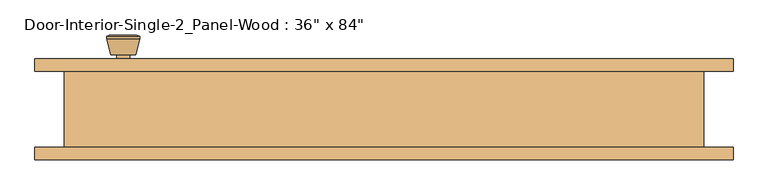
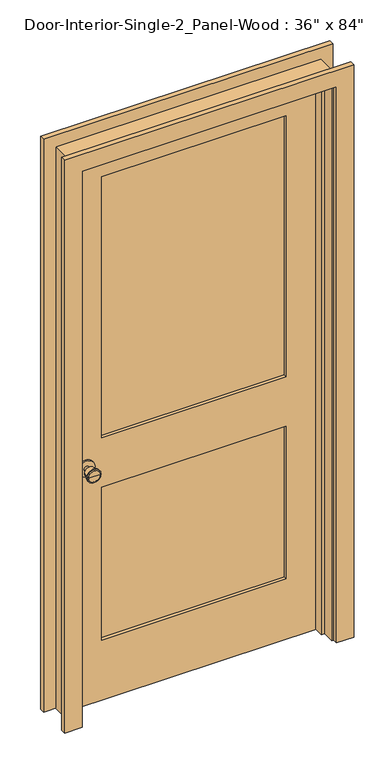
"""IFC4 building model written with IfcOpenShell, lengths in millimetres: door geometry."""

from ifc_helpers import new_model, si_unit, point, frame, frame_2d, origin, place, context, project, spatial, polyline, circle_curve, trimmed, segment, composite_curve, outline, extrude, faceted_brep, source, transform, mapped, element, save
from ifc_brep_helpers import plane_surface, cylinder_surface, revolved_surface, advanced_brep


def door_d4071c8b(model_context):
    return source(origin(), model_context, "Body", "SolidModel", [
        advanced_brep(
        [(-393.7, 13.05, 914.4), (-383.7, 13.05, 914.4), (-403.7, 13.05, 914.4), (-373.2241324, -35.95, 914.4), (-393.7, -35.95, 914.4), (-414.1758676, -35.95, 914.4), (-368.7, -34.1221319, 914.4), (-418.7, -34.1221319, 914.4), (-368.7, -30.6584537, 914.4), (-418.7, -30.6584537, 914.4), (-375.063764, -5.95, 914.4), (-412.336236, -5.95, 914.4), (-383.7, -5.95, 914.4), (-403.7, -5.95, 914.4)],
        [
            (0, 1),
            (1, 2, circle_curve(frame((-393.7, 13.05, 914.4), z_axis=(0.0, 1.0, 0.0), x_axis=(-1.0, 0.0, 0.0)), 10.0)),
            (2, 0),
            (2, 1, circle_curve(frame((-393.7, 13.05, 914.4), z_axis=(0.0, 1.0, 0.0), x_axis=(-1.0, 0.0, 0.0)), 10.0)),
            (3, 4),
            (4, 5),
            (5, 3, circle_curve(frame((-393.7, -35.95, 914.4), z_axis=(0.0, -1.0, 0.0), x_axis=(-1.0, 0.0, 0.0)), 20.4758676)),
            (3, 5, circle_curve(frame((-393.7, -35.95, 914.4), z_axis=(0.0, -1.0, 0.0), x_axis=(-1.0, 0.0, 0.0)), 20.4758676)),
            (6, 3),
            (5, 7),
            (7, 6, circle_curve(frame((-393.7, -34.1221319, 914.4), z_axis=(0.0, -1.0, 0.0), x_axis=(-1.0, 0.0, 0.0)), 25.0)),
            (6, 7, circle_curve(frame((-393.7, -34.1221319, 914.4), z_axis=(0.0, -1.0, 0.0), x_axis=(-1.0, 0.0, 0.0)), 25.0)),
            (8, 6),
            (7, 9),
            (9, 8, circle_curve(frame((-393.7, -30.6584537, 914.4), z_axis=(0.0, -1.0, 0.0), x_axis=(-1.0, 0.0, 0.0)), 25.0)),
            (8, 9, circle_curve(frame((-393.7, -30.6584537, 914.4), z_axis=(0.0, -1.0, 0.0), x_axis=(-1.0, 0.0, 0.0)), 25.0)),
            (10, 8),
            (9, 11),
            (11, 10, circle_curve(frame((-393.7, -5.95, 914.4), z_axis=(0.0, -1.0, 0.0), x_axis=(-1.0, 0.0, 0.0)), 18.636236)),
            (10, 11, circle_curve(frame((-393.7, -5.95, 914.4), z_axis=(0.0, -1.0, 0.0), x_axis=(-1.0, 0.0, 0.0)), 18.636236)),
            (12, 10),
            (11, 13),
            (13, 12, circle_curve(frame((-393.7, -5.95, 914.4), z_axis=(0.0, -1.0, 0.0), x_axis=(-1.0, 0.0, 0.0)), 10.0)),
            (12, 13, circle_curve(frame((-393.7, -5.95, 914.4), z_axis=(0.0, -1.0, 0.0), x_axis=(-1.0, 0.0, 0.0)), 10.0)),
            (1, 12),
            (13, 2),
        ],
        [
            plane_surface(frame((-393.7, 13.05, 914.4), z_axis=(0.0, 1.0, 0.0), x_axis=(-1.0, 0.0, 0.0))),
            plane_surface(frame((-393.7, -35.95, 914.4), z_axis=(0.0, -1.0, 0.0), x_axis=(-1.0, 0.0, 0.0))),
            revolved_surface(polyline([(-414.1758676, -35.95, 914.4), (-418.7, -34.1221319, 914.4)]), (-393.7, 13.05, 914.4), (0.0, 1.0, 0.0)),
            cylinder_surface(frame((-393.7, 13.05, 914.4), z_axis=(0.0, 1.0, 0.0), x_axis=(-1.0, 0.0, 0.0)), 25.0),
            revolved_surface(polyline([(-418.7, -30.6584537, 914.4), (-412.336236, -5.95, 914.4)]), (-393.7, 13.05, 914.4), (0.0, 1.0, 0.0)),
            plane_surface(frame((-393.7, -5.95, 914.4), z_axis=(0.0, 1.0, 0.0), x_axis=(-1.0, 0.0, 0.0))),
            cylinder_surface(frame((-393.7, 13.05, 914.4), z_axis=(0.0, 1.0, 0.0), x_axis=(-1.0, 0.0, 0.0)), 10.0),
        ],
        [
            (0, [[1, 2, 3]]),
            (0, [[-3, 4, -1]]),
            (1, [[5, 6, 7]]),
            (1, [[-6, -5, 8]]),
            (2, [[9, -7, 10, 11]]),
            (2, [[-10, -8, -9, 12]]),
            (3, [[13, -11, 14, 15]]),
            (3, [[-14, -12, -13, 16]]),
            (4, [[17, -15, 18, 19]]),
            (4, [[-18, -16, -17, 20]]),
            (5, [[21, -19, 22, 23]]),
            (5, [[-22, -20, -21, 24]]),
            (6, [[25, -23, 26, -2]]),
            (6, [[-26, -24, -25, -4]]),
        ],
    ),
        extrude(outline(composite_curve([segment(trimmed(circle_curve(frame_2d((914.4, -393.7)), 30.0), [point((914.4, -423.7))], [point((914.4, -363.7))], False, "CARTESIAN"), True, "CONTINUOUS"), segment(trimmed(circle_curve(frame_2d((914.4, -393.7)), 30.0), [point((914.4, -363.7))], [point((914.4, -423.7))], False, "CARTESIAN"), True, "CONTINUOUS")], self_intersect=False)), frame((0.0, 13.05, 0.0), z_axis=(0.0, 1.0, 0.0), x_axis=(0.0, 0.0, 1.0)), (0.0, 0.0, 1.0), 6.0),
        advanced_brep(
        [(-393.7, 59.975, 914.4), (-403.7, 59.975, 914.4), (-383.7, 59.975, 914.4), (-373.2241324, 108.975, 914.4), (-414.1758676, 108.975, 914.4), (-393.7, 108.975, 914.4), (-368.7, 107.1471319, 914.4), (-418.7, 107.1471319, 914.4), (-368.7, 103.6834537, 914.4), (-418.7, 103.6834537, 914.4), (-375.063764, 78.975, 914.4), (-412.336236, 78.975, 914.4), (-383.7, 78.975, 914.4), (-403.7, 78.975, 914.4)],
        [
            (0, 1),
            (1, 2, circle_curve(frame((-393.7, 59.975, 914.4), z_axis=(0.0, -1.0, 0.0), x_axis=(-1.0, 0.0, 0.0)), 10.0)),
            (2, 0),
            (2, 1, circle_curve(frame((-393.7, 59.975, 914.4), z_axis=(0.0, -1.0, 0.0), x_axis=(-1.0, 0.0, 0.0)), 10.0)),
            (3, 4, circle_curve(frame((-393.7, 108.975, 914.4), z_axis=(0.0, 1.0, 0.0), x_axis=(-1.0, 0.0, 0.0)), 20.4758676)),
            (4, 5),
            (5, 3),
            (4, 3, circle_curve(frame((-393.7, 108.975, 914.4), z_axis=(0.0, 1.0, 0.0), x_axis=(-1.0, 0.0, 0.0)), 20.4758676)),
            (6, 7, circle_curve(frame((-393.7, 107.1471319, 914.4), z_axis=(0.0, 1.0, 0.0), x_axis=(-1.0, 0.0, 0.0)), 25.0)),
            (7, 4),
            (3, 6),
            (7, 6, circle_curve(frame((-393.7, 107.1471319, 914.4), z_axis=(0.0, 1.0, 0.0), x_axis=(-1.0, 0.0, 0.0)), 25.0)),
            (8, 9, circle_curve(frame((-393.7, 103.6834537, 914.4), z_axis=(0.0, 1.0, 0.0), x_axis=(-1.0, 0.0, 0.0)), 25.0)),
            (9, 7),
            (6, 8),
            (9, 8, circle_curve(frame((-393.7, 103.6834537, 914.4), z_axis=(0.0, 1.0, 0.0), x_axis=(-1.0, 0.0, 0.0)), 25.0)),
            (10, 11, circle_curve(frame((-393.7, 78.975, 914.4), z_axis=(0.0, 1.0, 0.0), x_axis=(-1.0, 0.0, 0.0)), 18.636236)),
            (11, 9),
            (8, 10),
            (11, 10, circle_curve(frame((-393.7, 78.975, 914.4), z_axis=(0.0, 1.0, 0.0), x_axis=(-1.0, 0.0, 0.0)), 18.636236)),
            (12, 13, circle_curve(frame((-393.7, 78.975, 914.4), z_axis=(0.0, 1.0, 0.0), x_axis=(-1.0, 0.0, 0.0)), 10.0)),
            (13, 11),
            (10, 12),
            (13, 12, circle_curve(frame((-393.7, 78.975, 914.4), z_axis=(0.0, 1.0, 0.0), x_axis=(-1.0, 0.0, 0.0)), 10.0)),
            (1, 13),
            (12, 2),
        ],
        [
            plane_surface(frame((-393.7, 59.975, 914.4), z_axis=(0.0, -1.0, 0.0), x_axis=(-1.0, 0.0, 0.0))),
            plane_surface(frame((-393.7, 108.975, 914.4), z_axis=(0.0, 1.0, 0.0), x_axis=(-1.0, 0.0, 0.0))),
            revolved_surface(polyline([(-414.1758676, 108.975, 914.4), (-418.7, 107.1471319, 914.4)]), (-393.7, 59.975, 914.4), (0.0, -1.0, 0.0)),
            cylinder_surface(frame((-393.7, 59.975, 914.4), z_axis=(0.0, -1.0, 0.0), x_axis=(-1.0, 0.0, 0.0)), 25.0),
            revolved_surface(polyline([(-418.7, 103.6834537, 914.4), (-412.336236, 78.975, 914.4)]), (-393.7, 59.975, 914.4), (0.0, -1.0, 0.0)),
            plane_surface(frame((-393.7, 78.975, 914.4), z_axis=(0.0, -1.0, 0.0), x_axis=(-1.0, 0.0, 0.0))),
            cylinder_surface(frame((-393.7, 59.975, 914.4), z_axis=(0.0, -1.0, 0.0), x_axis=(-1.0, 0.0, 0.0)), 10.0),
        ],
        [
            (0, [[1, 2, 3]]),
            (0, [[-3, 4, -1]]),
            (1, [[5, 6, 7]]),
            (1, [[8, -7, -6]]),
            (2, [[9, 10, -5, 11]]),
            (2, [[12, -11, -8, -10]]),
            (3, [[13, 14, -9, 15]]),
            (3, [[16, -15, -12, -14]]),
            (4, [[17, 18, -13, 19]]),
            (4, [[20, -19, -16, -18]]),
            (5, [[21, 22, -17, 23]]),
            (5, [[24, -23, -20, -22]]),
            (6, [[-2, 25, -21, 26]]),
            (6, [[-4, -26, -24, -25]]),
        ],
    ),
        extrude(outline(composite_curve([segment(trimmed(circle_curve(frame_2d((914.4, -393.7)), 30.0), [point((914.4, -423.7))], [point((914.4, -363.7))], False, "CARTESIAN"), True, "CONTINUOUS"), segment(trimmed(circle_curve(frame_2d((914.4, -393.7)), 30.0), [point((914.4, -363.7))], [point((914.4, -423.7))], False, "CARTESIAN"), True, "CONTINUOUS")], self_intersect=False)), frame((0.0, 53.975, 0.0), z_axis=(0.0, 1.0, 0.0), x_axis=(0.0, 0.0, 1.0)), (0.0, 0.0, 1.0), 6.0),
        faceted_brep([(482.6, 53.975, 0.0), (482.6, -60.325, 0.0), (457.2, -60.325, 0.0), (457.2, -15.875, 0.0), (444.5, -15.875, 0.0), (444.5, 19.05, 0.0), (457.2, 19.05, 0.0), (457.2, 53.975, 0.0), (482.6, 53.975, 2159.0), (482.6, -60.325, 2159.0), (-482.6, -60.325, 2159.0), (-482.6, -60.325, 0.0), (-457.2, -60.325, 0.0), (-457.2, -60.325, 2133.6), (457.2, -60.325, 2133.6), (457.2, -15.875, 2133.6), (-457.2, -15.875, 2133.6), (-457.2, -15.875, 0.0), (-444.5, -15.875, 0.0), (-444.5, -15.875, 2120.9), (444.5, -15.875, 2120.9), (444.5, 19.05, 2120.9), (-444.5, 19.05, 2120.9), (-444.5, 19.05, 0.0), (-457.2, 19.05, 0.0), (-457.2, 19.05, 2133.6), (457.2, 19.05, 2133.6), (457.2, 53.975, 2133.6), (-457.2, 53.975, 2133.6), (-457.2, 53.975, 0.0), (-482.6, 53.975, 0.0), (-482.6, 53.975, 2159.0)], [[[0, 1, 2, 3, 4, 5, 6, 7]], [[1, 0, 8, 9]], [[2, 1, 9, 10, 11, 12, 13, 14]], [[3, 2, 14, 15]], [[4, 3, 15, 16, 17, 18, 19, 20]], [[5, 4, 20, 21]], [[6, 5, 21, 22, 23, 24, 25, 26]], [[7, 6, 26, 27]], [[0, 7, 27, 28, 29, 30, 31, 8]], [[9, 8, 31, 10]], [[15, 14, 13, 16]], [[21, 20, 19, 22]], [[27, 26, 25, 28]], [[30, 29, 24, 23, 18, 17, 12, 11]], [[10, 31, 30, 11]], [[16, 13, 12, 17]], [[22, 19, 18, 23]], [[28, 25, 24, 29]]]),
        extrude(outline(polyline([(2133.6, -457.2), (0.0, -457.2), (0.0, 457.2), (2133.6, 457.2), (2133.6, -457.2)]), holes=[polyline([(2014.5375, -336.55), (2014.5375, 336.55), (1009.65, 336.55), (1009.65, -336.55), (2014.5375, -336.55)]), polyline([(819.15, -336.55), (819.15, 336.55), (231.775, 336.55), (231.775, -336.55), (819.15, -336.55)])]), frame((0.0, 19.05, 0.0), z_axis=(0.0, 1.0, 0.0), x_axis=(0.0, 0.0, 1.0)), (0.0, 0.0, 1.0), 34.925),
        extrude(outline(polyline([(336.55, 30.6916667), (-336.55, 30.6916667), (-336.55, 42.3333333), (336.55, 42.3333333), (336.55, 30.6916667)])), frame((0.0, 0.0, 1009.65), z_axis=(0.0, 0.0, 1.0), x_axis=(1.0, 0.0, 0.0)), (0.0, 0.0, 1.0), 1004.8875),
        extrude(outline(polyline([(336.55, 30.6916667), (-336.55, 30.6916667), (-336.55, 42.3333333), (336.55, 42.3333333), (336.55, 30.6916667)])), frame((0.0, 0.0, 231.775), z_axis=(0.0, 0.0, 1.0), x_axis=(1.0, 0.0, 0.0)), (0.0, 0.0, 1.0), 587.375),
        extrude(outline(polyline([(0.0, 463.55), (0.0, 527.05), (2203.45, 527.05), (2203.45, -527.05), (0.0, -527.05), (0.0, -463.55), (2139.95, -463.55), (2139.95, 463.55), (0.0, 463.55)])), frame((0.0, 53.975, 0.0), z_axis=(0.0, 1.0, 0.0), x_axis=(0.0, 0.0, 1.0)), (0.0, 0.0, 1.0), 19.05),
        extrude(outline(polyline([(0.0, 463.55), (0.0, 527.05), (2203.45, 527.05), (2203.45, -527.05), (0.0, -527.05), (0.0, -463.55), (2139.95, -463.55), (2139.95, 463.55), (0.0, 463.55)])), frame((0.0, -79.375, 0.0), z_axis=(0.0, 1.0, 0.0), x_axis=(0.0, 0.0, 1.0)), (0.0, 0.0, 1.0), 19.05),
    ])


if __name__ == "__main__":
    model = new_model("IFC4")
    model_context = context("Model", 3, world=origin())
    ifc_project = project(units=[si_unit("LENGTHUNIT", "METRE", prefix="MILLI")], contexts=[model_context])
    site = spatial("IfcSite", under=ifc_project)
    building = spatial("IfcBuilding", under=site)
    placement = place(None, origin())
    door_shape = door_d4071c8b(model_context)
    element("IfcDoor", 1, ObjectType="Door-Interior-Single-2_Panel-Wood : 36\" x 84\"", at=placement, inside=building, context=model_context, shape_type="MappedRepresentation", body=[
        mapped(door_shape, transform((0.0, 0.0, 0.0), x_axis=(1.0, 0.0, 0.0), y_axis=(0.0, 1.0, 0.0), z_axis=(0.0, 0.0, 1.0))),
    ])
    save(model, "model.ifc")

# Revit data of these elements
# Type "Door-Interior-Single-2_Panel-Wood : 36\" x 84\""
#   Type Mark = "9"
#   Assembly Code = "C1020300"
#   Analytic Construction = "Wooden"
#   Top Rail = 0' - 4 11/16"
#   Thickness = 0' - 1 3/8"
#   Thermal Resistance (R) = 2.5876 (h·ft²·°F)/BTU
#   Swing Angle [instance default] = 90.00°
#   Stiles = 0' - 4 3/4"
#   Rough Width = 3' - 2"
#   Rough Height = 7' - 1"
#   Lock Rail = 0' - 7 1/2"
#   Height = 7' - 0"
#   Width = 3' - 0"
#   Heat Transfer Coefficient (U) = 0.3865 BTU/(h·ft²·°F)
#   Bottom Rail = 0' - 9 1/8"
#   Trim Material = Cherry
#   Panel Material = Cherry
#   Frame Material = Cherry
#   Door Handle Material = Aluminum
#   Visual Light Transmittance = 0
#   Solar Heat Gain Coefficient = 0
#   Wall Closure = (empty or 0)
#   Function = (empty or 0)
# Element 1 (IfcDoor, "Door-Interior-Single-2_Panel-Wood : 36\" x 84\"")
#   Materials on its faces: "Cherry", "Aluminum"
# Materials
#   "Cherry": class "Wood", colour RGB 226 177 128, transparency 0, Description = "Prunus Serotina", Cost = 0
#   "Aluminum": class "Metal", colour RGB 247 247 247, transparency 0, Description = "Aluminum 6061", Cost = 0
